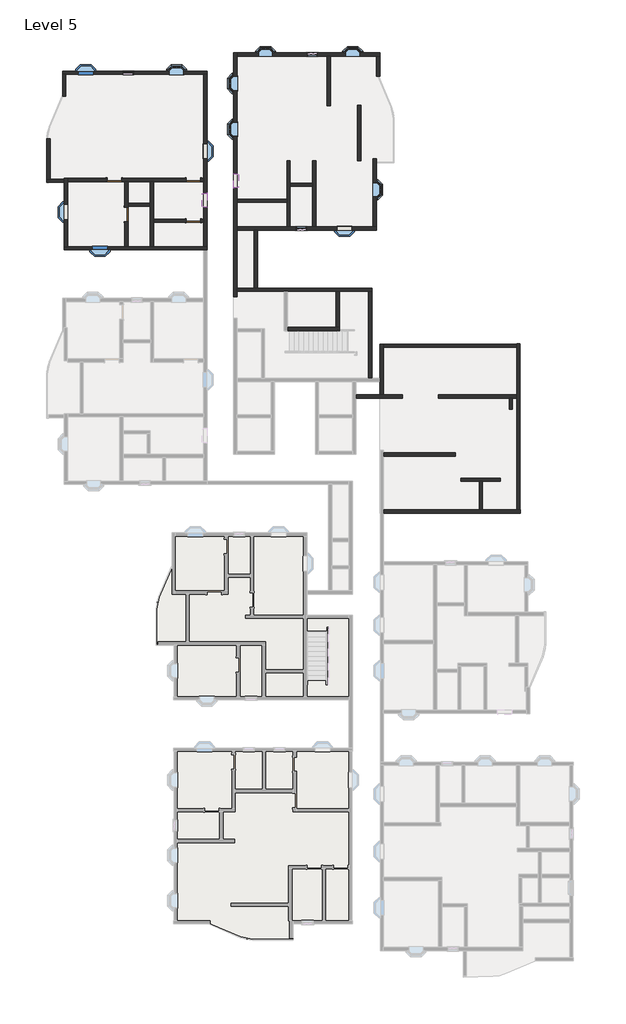
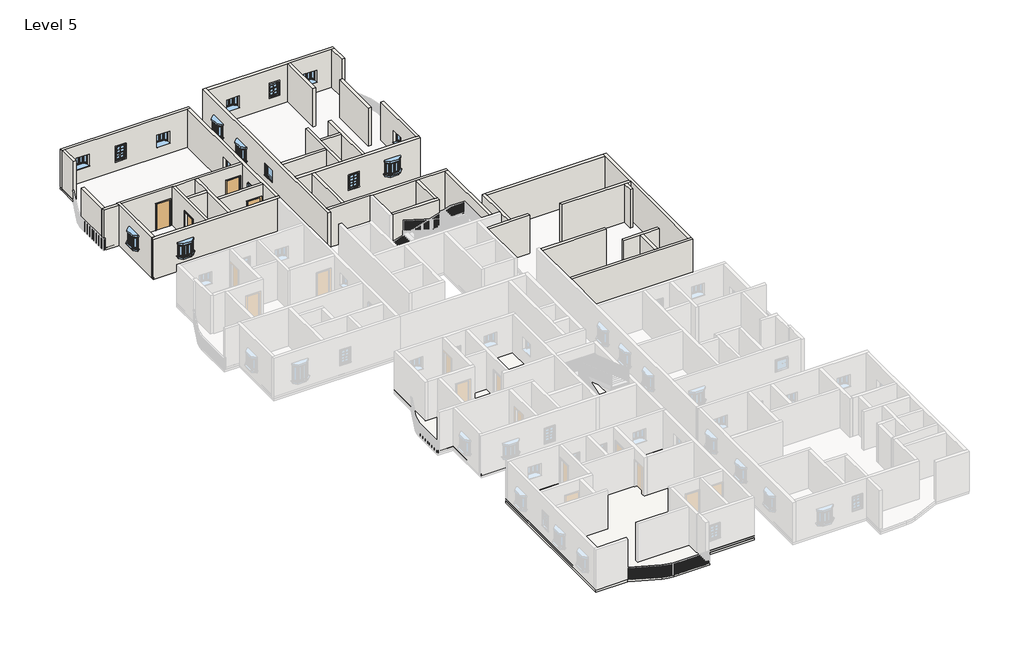
# One storey, part 4 of 14: 38 walls, 16 windows, 4 doors, 2 roofs, 1 slab.
# Revit data of these elements (continued)
# Elements 30, 37, 38, 39, 40 (IfcWall, "9\" w")
#   Top Offset = 0' - 0"
#   Base Offset = 0' - 0"
#   wall height = 10' - 0"
#   Phase Created = New Construction
#   Base Constraint = Level 5
#   Top Constraint = Level 6
#   Materials on its faces: "Default Wall"
# Elements 31, 43 (IfcWall, "9\" w")
#   Top Offset = 0' - 0"
#   Base Offset = 0' - 0"
#   wall height = 10' - 0"
#   Phase Created = New Construction
#   Base Constraint = Level 5
#   Top Constraint = Level 6
#   Materials on its faces: "Default Wall", "Brick, Soldier Course"
# Element 32 (IfcWall, "9\" w")
#   Top Offset = 0' - 0"
#   Base Offset = 0' - 0"
#   wall height = 10' - 0"
#   Phase Created = New Construction
#   Base Constraint = Level 5
#   Top Constraint = Level 6
#   Materials on its faces: "Default Wall", "Brick, Soldier Course", "Earth"
# Element 33 (IfcWall, "9\" w")
#   Top Offset = 0' - 0"
#   Base Offset = 0' - 0"
#   wall height = 10' - 0"
#   Phase Created = New Construction
#   Base Constraint = Level 5
#   Top Constraint = Level 6
#   Materials on its faces: "Default Wall", "Earth"
# Elements 34, 35, 36 (IfcWall, "9\" w")
#   Top Offset = 0' - 0"
#   Base Offset = 0' - 0"
#   wall height = 10' - 0"
#   Phase Created = New Construction
#   Base Constraint = Level 5
#   Top Constraint = Level 6
#   Materials on its faces: "Default Wall", "Window Frame"
# Element 41 (IfcWall, "9\" w")
#   Top Offset = 0' - 0"
#   Base Offset = 0' - 0"
#   wall height = 10' - 0"
#   Phase Created = New Construction
#   Base Constraint = Level 5
#   Top Constraint = Level 6
#   Materials on its faces: "Default Wall", "Parking Stripe", "Default Mass Interior Wall"
# Element 42 (IfcWall, "9\" w")
#   Top Offset = 0' - 0"
#   Base Offset = 0' - 0"
#   wall height = 10' - 0"
#   Phase Created = New Construction
#   Base Constraint = Level 5
#   Top Constraint = Level 6
#   Materials on its faces: "Default Wall", "Parking Stripe", "Brick, Soldier Course"
# Element 44 (IfcWall, "9\" w")
#   Top Offset = 0' - 0"
#   Base Offset = 0' - 0"
#   wall height = 10' - 0"
#   Phase Created = New Construction
#   Base Constraint = Level 5
#   Top Constraint = Level 6
#   Materials on its faces: "Default Wall", "Parking Stripe"
# Element 45 (IfcWall, "9\" w")
#   Top Offset = 0' - 0"
#   Base Offset = 0' - 0"
#   wall height = 10' - 0"
#   Phase Created = New Construction
#   Base Constraint = Level 5
#   Top Constraint = Level 6
#   Materials on its faces: "Default Wall", "Grass"
# Element 46 (IfcWindow, "910x910mm")
#   Mark = "224"
#   Phase Created = New Construction
#   Materials on its faces: "Window Frame", "Glass"
# Element 47 (IfcWindow, "910x910mm")
#   Mark = "225"
#   Phase Created = New Construction
#   Materials on its faces: "Window Frame", "Glass"
# Element 48 (IfcWindow, "910x910mm")
#   Mark = "286"
#   Phase Created = New Construction
#   Materials on its faces: "Window Frame", "Glass"
# Element 49 (IfcWindow, "910x910mm")
#   Mark = "287"
#   Phase Created = New Construction
#   Materials on its faces: "Window Frame", "Glass"
# Element 50 (IfcWindow, "910x910mm")
#   Mark = "298"
#   Phase Created = New Construction
#   Materials on its faces: "Window Frame", "Glass"
# Element 51 (IfcWindow, "910x910mm")
#   Mark = "299"
#   Phase Created = New Construction
#   Materials on its faces: "Window Frame", "Glass"
# Element 52 (IfcWindow, "910x910mm")
#   Mark = "493"
#   Phase Created = New Construction
#   Materials on its faces: "Window Frame", "Glass"
# Element 53 (IfcWindow, "910x910mm")
#   Mark = "494"
#   Phase Created = New Construction
#   Materials on its faces: "Window Frame", "Glass"
# Element 54 (IfcWindow, "910x910mm")
#   Mark = "498"
#   Phase Created = New Construction
#   Materials on its faces: "Window Frame", "Glass"
# Element 55 (IfcWindow, "910x910mm")
#   Mark = "257"
#   Phase Created = New Construction
#   Materials on its faces: "Window Frame", "Glass"
# Element 56 (IfcWindow, "910x910mm")
#   Mark = "258"
#   Phase Created = New Construction
#   Materials on its faces: "Window Frame", "Glass"
# Element 57 (IfcWindow, "Window-Double-Hung : 26\" x 42\"")
#   Mark = "288"
#   Window Inset = 0' - 0"
#   Interior Wall Closure = 0' - 1 1/2"
#   Frame Extension = 0' - 1 1/4"
#   Exterior Wall Closure = 0' - 0 1/2"
#   Interior Trim Visibility = yes
#   Indicator Visibility = yes
#   Exterior Trim Visibility = yes
#   Phase Created = New Construction
#   Materials on its faces: "Wood - Stained", "Glass", "Clad - White"
# Element 58 (IfcWindow, "Window-Double-Hung : 26\" x 42\"")
#   Mark = "300"
#   Window Inset = 0' - 0"
#   Interior Wall Closure = 0' - 1 1/2"
#   Frame Extension = 0' - 1 1/4"
#   Exterior Wall Closure = 0' - 0 1/2"
#   Interior Trim Visibility = yes
#   Indicator Visibility = yes
#   Exterior Trim Visibility = yes
#   Phase Created = New Construction
#   Materials on its faces: "Wood - Stained", "Glass", "Clad - White"
# Element 59 (IfcWindow, "Window-Double-Hung : 26\" x 42\"")
#   Mark = "276"
#   Window Inset = 0' - 0"
#   Interior Wall Closure = 0' - 1 1/2"
#   Frame Extension = 0' - 1 1/4"
#   Exterior Wall Closure = 0' - 0 1/2"
#   Interior Trim Visibility = yes
#   Indicator Visibility = yes
#   Exterior Trim Visibility = yes
#   Phase Created = New Construction
#   Materials on its faces: "Wood - Stained", "Glass", "Clad - White"
# Element 60 (IfcWindow, "Windows_Sgl_w-Glazing_Bars : 910x910mm")
#   Mark = "495"
#   Phase Created = New Construction
#   Materials on its faces: "Window Frame", "Glass"
# Element 61 (IfcWindow, "Windows_Sgl_w-Glazing_Bars : 910x910mm")
#   Mark = "499"
#   Phase Created = New Construction
#   Materials on its faces: "Window Frame", "Glass"
# Materials
#   "Door - Panel": class "Wood", colour RGB 210 159 95, transparency 0, Cost = 0
#   "Door - Frame": colour RGB 118 70 51, transparency 0, Cost = 0
#   "Window Frame": colour RGB 249 249 249, transparency 0
#   "Glass": class "Glass", colour RGB 0 128 192, transparency 0.75, Description = "Soda Lime Glass", Cost = 0
#   "Wood - Stained": class "Wood", colour RGB 224 178 126, transparency 0, Cost = 0
#   "Clad - White": class "Wood", colour RGB 242 242 238, transparency 0, Cost = 0
#   "Default Roof": colour RGB 88 101 114, transparency 0, Cost = 0
#   "Default Floor": colour RGB 128 128 128, transparency 0, Cost = 0
#   "Default Wall": colour RGB 128 128 128, transparency 0, Cost = 0
#   "Parking Stripe": class "Paint", colour RGB 250 250 91, transparency 0, Cost = 0
#   "Carpet (1)": class "Carpet", colour RGB 124 80 67, transparency 0, Description = "Interior finish", Cost = 0
#   "Brick, Soldier Course": class "Masonry", colour RGB 170 98 104, transparency 0, Description = "Common brick soldier coursed", Cost = 0
#   "Default Mass Interior Wall": class "Generic", colour RGB 195 229 126, transparency 0, Cost = 0
#   "Earth": class "Generic", colour RGB 97 75 62, transparency 0, Description = "Soil", Cost = 0
#   "Grass": class "Generic", colour RGB 104 137 66, transparency 0, Description = "Physical material.", Cost = 0
